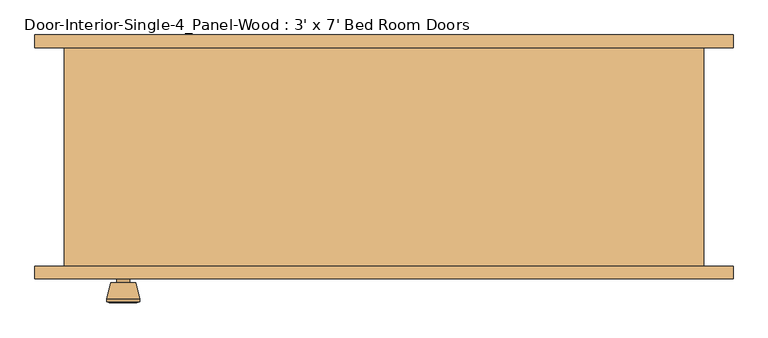
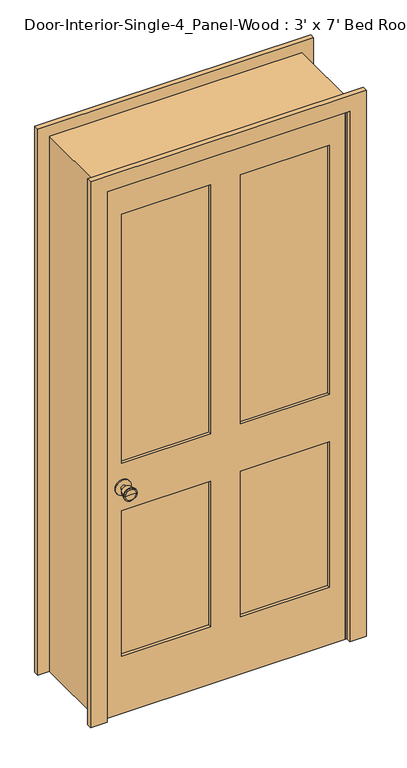
"""IFC4 building model written with IfcOpenShell, lengths in millimetres: door geometry, Door-Interior-Single-4_Panel-Wood : 3' x 7' Bed Room Doors."""

from ifc_helpers import new_model, si_unit, point, frame, frame_2d, origin, place, context, project, spatial, polyline, circle_curve, trimmed, segment, composite_curve, outline, extrude, faceted_brep, source, transform, mapped, element, save
from ifc_brep_helpers import plane_surface, cylinder_surface, revolved_surface, advanced_brep


def door_interior_single_4_panel_wood_3_x_7_bed_room_doors_8c54f457(model_context):
    return source(origin(), model_context, "Body", "SolidModel", [
        advanced_brep(
        [(-393.7, -121.0, 914.4), (-403.7, -121.0, 914.4), (-383.7, -121.0, 914.4), (-373.2241324, -72.0, 914.4), (-414.1758676, -72.0, 914.4), (-393.7, -72.0, 914.4), (-368.7, -73.8278681, 914.4), (-418.7, -73.8278681, 914.4), (-368.7, -77.2915463, 914.4), (-418.7, -77.2915463, 914.4), (-375.063764, -102.0, 914.4), (-412.336236, -102.0, 914.4), (-383.7, -102.0, 914.4), (-403.7, -102.0, 914.4)],
        [
            (0, 1),
            (1, 2, circle_curve(frame((-393.7, -121.0, 914.4), z_axis=(0.0, -1.0, 0.0), x_axis=(-1.0, 0.0, 0.0)), 10.0)),
            (2, 0),
            (2, 1, circle_curve(frame((-393.7, -121.0, 914.4), z_axis=(0.0, -1.0, 0.0), x_axis=(-1.0, 0.0, 0.0)), 10.0)),
            (3, 4, circle_curve(frame((-393.7, -72.0, 914.4), z_axis=(0.0, 1.0, 0.0), x_axis=(-1.0, 0.0, 0.0)), 20.4758676)),
            (4, 5),
            (5, 3),
            (4, 3, circle_curve(frame((-393.7, -72.0, 914.4), z_axis=(0.0, 1.0, 0.0), x_axis=(-1.0, 0.0, 0.0)), 20.4758676)),
            (6, 7, circle_curve(frame((-393.7, -73.8278681, 914.4), z_axis=(0.0, 1.0, 0.0), x_axis=(-1.0, 0.0, 0.0)), 25.0)),
            (7, 4),
            (3, 6),
            (7, 6, circle_curve(frame((-393.7, -73.8278681, 914.4), z_axis=(0.0, 1.0, 0.0), x_axis=(-1.0, 0.0, 0.0)), 25.0)),
            (8, 9, circle_curve(frame((-393.7, -77.2915463, 914.4), z_axis=(0.0, 1.0, 0.0), x_axis=(-1.0, 0.0, 0.0)), 25.0)),
            (9, 7),
            (6, 8),
            (9, 8, circle_curve(frame((-393.7, -77.2915463, 914.4), z_axis=(0.0, 1.0, 0.0), x_axis=(-1.0, 0.0, 0.0)), 25.0)),
            (10, 11, circle_curve(frame((-393.7, -102.0, 914.4), z_axis=(0.0, 1.0, 0.0), x_axis=(-1.0, 0.0, 0.0)), 18.636236)),
            (11, 9),
            (8, 10),
            (11, 10, circle_curve(frame((-393.7, -102.0, 914.4), z_axis=(0.0, 1.0, 0.0), x_axis=(-1.0, 0.0, 0.0)), 18.636236)),
            (12, 13, circle_curve(frame((-393.7, -102.0, 914.4), z_axis=(0.0, 1.0, 0.0), x_axis=(-1.0, 0.0, 0.0)), 10.0)),
            (13, 11),
            (10, 12),
            (13, 12, circle_curve(frame((-393.7, -102.0, 914.4), z_axis=(0.0, 1.0, 0.0), x_axis=(-1.0, 0.0, 0.0)), 10.0)),
            (1, 13),
            (12, 2),
        ],
        [
            plane_surface(frame((-393.7, -121.0, 914.4), z_axis=(0.0, -1.0, 0.0), x_axis=(-1.0, 0.0, 0.0))),
            plane_surface(frame((-393.7, -72.0, 914.4), z_axis=(0.0, 1.0, 0.0), x_axis=(-1.0, 0.0, 0.0))),
            revolved_surface(polyline([(-414.1758676, -72.0, 914.4), (-418.7, -73.8278681, 914.4)]), (-393.7, -121.0, 914.4), (0.0, -1.0, 0.0)),
            cylinder_surface(frame((-393.7, -121.0, 914.4), z_axis=(0.0, -1.0, 0.0), x_axis=(-1.0, 0.0, 0.0)), 25.0),
            revolved_surface(polyline([(-418.7, -77.2915463, 914.4), (-412.336236, -102.0, 914.4)]), (-393.7, -121.0, 914.4), (0.0, -1.0, 0.0)),
            plane_surface(frame((-393.7, -102.0, 914.4), z_axis=(0.0, -1.0, 0.0), x_axis=(-1.0, 0.0, 0.0))),
            cylinder_surface(frame((-393.7, -121.0, 914.4), z_axis=(0.0, -1.0, 0.0), x_axis=(-1.0, 0.0, 0.0)), 10.0),
        ],
        [
            (0, [[1, 2, 3]]),
            (0, [[-3, 4, -1]]),
            (1, [[5, 6, 7]]),
            (1, [[8, -7, -6]]),
            (2, [[9, 10, -5, 11]]),
            (2, [[12, -11, -8, -10]]),
            (3, [[13, 14, -9, 15]]),
            (3, [[16, -15, -12, -14]]),
            (4, [[17, 18, -13, 19]]),
            (4, [[20, -19, -16, -18]]),
            (5, [[21, 22, -17, 23]]),
            (5, [[24, -23, -20, -22]]),
            (6, [[-2, 25, -21, 26]]),
            (6, [[-4, -26, -24, -25]]),
        ],
    ),
        extrude(outline(composite_curve([segment(trimmed(circle_curve(frame_2d((914.4, -393.7)), 30.0), [point((914.4, -423.7))], [point((914.4, -363.7))], False, "CARTESIAN"), True, "CONTINUOUS"), segment(trimmed(circle_curve(frame_2d((914.4, -393.7)), 30.0), [point((914.4, -363.7))], [point((914.4, -423.7))], False, "CARTESIAN"), True, "CONTINUOUS")], self_intersect=False)), frame((0.0, -127.0, 0.0), z_axis=(0.0, 1.0, 0.0), x_axis=(0.0, 0.0, 1.0)), (0.0, 0.0, 1.0), 6.0),
        advanced_brep(
        [(-393.7, -167.925, 914.4), (-383.7, -167.925, 914.4), (-403.7, -167.925, 914.4), (-373.2241324, -216.925, 914.4), (-393.7, -216.925, 914.4), (-414.1758676, -216.925, 914.4), (-368.7, -215.0971319, 914.4), (-418.7, -215.0971319, 914.4), (-368.7, -211.6334537, 914.4), (-418.7, -211.6334537, 914.4), (-375.063764, -186.925, 914.4), (-412.336236, -186.925, 914.4), (-383.7, -186.925, 914.4), (-403.7, -186.925, 914.4)],
        [
            (0, 1),
            (1, 2, circle_curve(frame((-393.7, -167.925, 914.4), z_axis=(0.0, 1.0, 0.0), x_axis=(-1.0, 0.0, 0.0)), 10.0)),
            (2, 0),
            (2, 1, circle_curve(frame((-393.7, -167.925, 914.4), z_axis=(0.0, 1.0, 0.0), x_axis=(-1.0, 0.0, 0.0)), 10.0)),
            (3, 4),
            (4, 5),
            (5, 3, circle_curve(frame((-393.7, -216.925, 914.4), z_axis=(0.0, -1.0, 0.0), x_axis=(-1.0, 0.0, 0.0)), 20.4758676)),
            (3, 5, circle_curve(frame((-393.7, -216.925, 914.4), z_axis=(0.0, -1.0, 0.0), x_axis=(-1.0, 0.0, 0.0)), 20.4758676)),
            (6, 3),
            (5, 7),
            (7, 6, circle_curve(frame((-393.7, -215.0971319, 914.4), z_axis=(0.0, -1.0, 0.0), x_axis=(-1.0, 0.0, 0.0)), 25.0)),
            (6, 7, circle_curve(frame((-393.7, -215.0971319, 914.4), z_axis=(0.0, -1.0, 0.0), x_axis=(-1.0, 0.0, 0.0)), 25.0)),
            (8, 6),
            (7, 9),
            (9, 8, circle_curve(frame((-393.7, -211.6334537, 914.4), z_axis=(0.0, -1.0, 0.0), x_axis=(-1.0, 0.0, 0.0)), 25.0)),
            (8, 9, circle_curve(frame((-393.7, -211.6334537, 914.4), z_axis=(0.0, -1.0, 0.0), x_axis=(-1.0, 0.0, 0.0)), 25.0)),
            (10, 8),
            (9, 11),
            (11, 10, circle_curve(frame((-393.7, -186.925, 914.4), z_axis=(0.0, -1.0, 0.0), x_axis=(-1.0, 0.0, 0.0)), 18.636236)),
            (10, 11, circle_curve(frame((-393.7, -186.925, 914.4), z_axis=(0.0, -1.0, 0.0), x_axis=(-1.0, 0.0, 0.0)), 18.636236)),
            (12, 10),
            (11, 13),
            (13, 12, circle_curve(frame((-393.7, -186.925, 914.4), z_axis=(0.0, -1.0, 0.0), x_axis=(-1.0, 0.0, 0.0)), 10.0)),
            (12, 13, circle_curve(frame((-393.7, -186.925, 914.4), z_axis=(0.0, -1.0, 0.0), x_axis=(-1.0, 0.0, 0.0)), 10.0)),
            (1, 12),
            (13, 2),
        ],
        [
            plane_surface(frame((-393.7, -167.925, 914.4), z_axis=(0.0, 1.0, 0.0), x_axis=(-1.0, 0.0, 0.0))),
            plane_surface(frame((-393.7, -216.925, 914.4), z_axis=(0.0, -1.0, 0.0), x_axis=(-1.0, 0.0, 0.0))),
            revolved_surface(polyline([(-414.1758676, -216.925, 914.4), (-418.7, -215.0971319, 914.4)]), (-393.7, -167.925, 914.4), (0.0, 1.0, 0.0)),
            cylinder_surface(frame((-393.7, -167.925, 914.4), z_axis=(0.0, 1.0, 0.0), x_axis=(-1.0, 0.0, 0.0)), 25.0),
            revolved_surface(polyline([(-418.7, -211.6334537, 914.4), (-412.336236, -186.925, 914.4)]), (-393.7, -167.925, 914.4), (0.0, 1.0, 0.0)),
            plane_surface(frame((-393.7, -186.925, 914.4), z_axis=(0.0, 1.0, 0.0), x_axis=(-1.0, 0.0, 0.0))),
            cylinder_surface(frame((-393.7, -167.925, 914.4), z_axis=(0.0, 1.0, 0.0), x_axis=(-1.0, 0.0, 0.0)), 10.0),
        ],
        [
            (0, [[1, 2, 3]]),
            (0, [[-3, 4, -1]]),
            (1, [[5, 6, 7]]),
            (1, [[-6, -5, 8]]),
            (2, [[9, -7, 10, 11]]),
            (2, [[-10, -8, -9, 12]]),
            (3, [[13, -11, 14, 15]]),
            (3, [[-14, -12, -13, 16]]),
            (4, [[17, -15, 18, 19]]),
            (4, [[-18, -16, -17, 20]]),
            (5, [[21, -19, 22, 23]]),
            (5, [[-22, -20, -21, 24]]),
            (6, [[25, -23, 26, -2]]),
            (6, [[-26, -24, -25, -4]]),
        ],
    ),
        extrude(outline(composite_curve([segment(trimmed(circle_curve(frame_2d((914.4, -393.7)), 30.0), [point((914.4, -423.7))], [point((914.4, -363.7))], False, "CARTESIAN"), True, "CONTINUOUS"), segment(trimmed(circle_curve(frame_2d((914.4, -393.7)), 30.0), [point((914.4, -363.7))], [point((914.4, -423.7))], False, "CARTESIAN"), True, "CONTINUOUS")], self_intersect=False)), frame((0.0, -167.925, 0.0), z_axis=(0.0, 1.0, 0.0), x_axis=(0.0, 0.0, 1.0)), (0.0, 0.0, 1.0), 6.0),
        faceted_brep([(482.6, -161.925, 0.0), (457.2, -161.925, 0.0), (457.2, -127.0, 0.0), (444.5, -127.0, 0.0), (444.5, -92.075, 0.0), (457.2, -92.075, 0.0), (457.2, 168.275, 0.0), (482.6, 168.275, 0.0), (482.6, 168.275, 2159.0), (482.6, -161.925, 2159.0), (457.2, 168.275, 2133.6), (-457.2, 168.275, 2133.6), (-457.2, 168.275, 0.0), (-482.6, 168.275, 0.0), (-482.6, 168.275, 2159.0), (457.2, -92.075, 2133.6), (444.5, -92.075, 2120.9), (-444.5, -92.075, 2120.9), (-444.5, -92.075, 0.0), (-457.2, -92.075, 0.0), (-457.2, -92.075, 2133.6), (444.5, -127.0, 2120.9), (457.2, -127.0, 2133.6), (-457.2, -127.0, 2133.6), (-457.2, -127.0, 0.0), (-444.5, -127.0, 0.0), (-444.5, -127.0, 2120.9), (457.2, -161.925, 2133.6), (-482.6, -161.925, 2159.0), (-482.6, -161.925, 0.0), (-457.2, -161.925, 0.0), (-457.2, -161.925, 2133.6)], [[[0, 1, 2, 3, 4, 5, 6, 7]], [[7, 8, 9, 0]], [[6, 10, 11, 12, 13, 14, 8, 7]], [[5, 15, 10, 6]], [[4, 16, 17, 18, 19, 20, 15, 5]], [[3, 21, 16, 4]], [[2, 22, 23, 24, 25, 26, 21, 3]], [[1, 27, 22, 2]], [[0, 9, 28, 29, 30, 31, 27, 1]], [[8, 14, 28, 9]], [[15, 20, 11, 10]], [[21, 26, 17, 16]], [[27, 31, 23, 22]], [[29, 13, 12, 19, 18, 25, 24, 30]], [[14, 13, 29, 28]], [[20, 19, 12, 11]], [[26, 25, 18, 17]], [[31, 30, 24, 23]]]),
        extrude(outline(polyline([(2133.6, -457.2), (0.0, -457.2), (0.0, 457.2), (2133.6, 457.2), (2133.6, -457.2)]), holes=[polyline([(2014.5375, 57.15), (2014.5375, 396.875), (1009.65, 396.875), (1009.65, 57.15), (2014.5375, 57.15)]), polyline([(1009.65, -57.15), (1009.65, -396.875), (2014.5375, -396.875), (2014.5375, -57.15), (1009.65, -57.15)]), polyline([(819.15, 57.15), (819.15, 396.875), (231.775, 396.875), (231.775, 57.15), (819.15, 57.15)]), polyline([(231.775, -57.15), (231.775, -396.875), (819.15, -396.875), (819.15, -57.15), (231.775, -57.15)])]), frame((0.0, -161.925, 0.0), z_axis=(0.0, 1.0, 0.0), x_axis=(0.0, 0.0, 1.0)), (0.0, 0.0, 1.0), 34.925),
        extrude(outline(polyline([(396.875, -138.6416667), (396.875, -150.2833333), (57.15, -150.2833333), (57.15, -138.6416667), (396.875, -138.6416667)])), frame((0.0, 0.0, 1009.65), z_axis=(0.0, 0.0, 1.0), x_axis=(1.0, 0.0, 0.0)), (0.0, 0.0, 1.0), 1004.8875),
        extrude(outline(polyline([(-57.15, -138.6416667), (-57.15, -150.2833333), (-396.875, -150.2833333), (-396.875, -138.6416667), (-57.15, -138.6416667)])), frame((0.0, 0.0, 1009.65), z_axis=(0.0, 0.0, 1.0), x_axis=(1.0, 0.0, 0.0)), (0.0, 0.0, 1.0), 1004.8875),
        extrude(outline(polyline([(396.875, -138.6416667), (396.875, -150.2833333), (57.15, -150.2833333), (57.15, -138.6416667), (396.875, -138.6416667)])), frame((0.0, 0.0, 231.775), z_axis=(0.0, 0.0, 1.0), x_axis=(1.0, 0.0, 0.0)), (0.0, 0.0, 1.0), 587.375),
        extrude(outline(polyline([(-57.15, -138.6416667), (-57.15, -150.2833333), (-396.875, -150.2833333), (-396.875, -138.6416667), (-57.15, -138.6416667)])), frame((0.0, 0.0, 231.775), z_axis=(0.0, 0.0, 1.0), x_axis=(1.0, 0.0, 0.0)), (0.0, 0.0, 1.0), 587.375),
        extrude(outline(polyline([(0.0, 527.05), (2203.45, 527.05), (2203.45, -527.05), (0.0, -527.05), (0.0, -463.55), (2139.95, -463.55), (2139.95, 463.55), (0.0, 463.55), (0.0, 527.05)])), frame((0.0, -180.975, 0.0), z_axis=(0.0, 1.0, 0.0), x_axis=(0.0, 0.0, 1.0)), (0.0, 0.0, 1.0), 19.05),
        extrude(outline(polyline([(0.0, 527.05), (2203.45, 527.05), (2203.45, -527.05), (0.0, -527.05), (0.0, -463.55), (2139.95, -463.55), (2139.95, 463.55), (0.0, 463.55), (0.0, 527.05)])), frame((0.0, 168.275, 0.0), z_axis=(0.0, 1.0, 0.0), x_axis=(0.0, 0.0, 1.0)), (0.0, 0.0, 1.0), 19.05),
    ])


if __name__ == "__main__":
    model = new_model("IFC4")
    model_context = context("Model", 3, world=origin())
    ifc_project = project(units=[si_unit("LENGTHUNIT", "METRE", prefix="MILLI")], contexts=[model_context])
    site = spatial("IfcSite", under=ifc_project)
    building = spatial("IfcBuilding", under=site)
    placement = place(None, origin())
    door_interior_single_4_panel_wood_3_x_7_bed_room_doors_shape = door_interior_single_4_panel_wood_3_x_7_bed_room_doors_8c54f457(model_context)
    element("IfcDoor", 1, ObjectType="Door-Interior-Single-4_Panel-Wood : 3' x 7' Bed Room Doors", at=placement, inside=building, context=model_context, shape_type="MappedRepresentation", body=[
        mapped(door_interior_single_4_panel_wood_3_x_7_bed_room_doors_shape, transform((0.0, 0.0, 0.0), x_axis=(1.0, 0.0, 0.0), y_axis=(0.0, 1.0, 0.0), z_axis=(0.0, 0.0, 1.0))),
    ])
    save(model, "model.ifc")

# Revit data of these elements
# Type "Door-Interior-Single-4_Panel-Wood : 3' x 7' Bed Room Doors"
#   Type Mark = "13"
#   Assembly Code = "C1020300"
#   Analytic Construction = "Wooden"
#   Top Rail = 0' - 4 11/16"
#   Thickness = 0' - 1 3/8"
#   Thermal Resistance (R) = 2.5876 (h·ft²·°F)/BTU
#   Swing Angle [instance default] = 90.00°
#   Stiles = 0' - 2 3/8"
#   Rough Width = 3' - 2"
#   Rough Height = 7' - 1"
#   Mullion = 0' - 4 1/2"
#   Lock Rail = 0' - 7 1/2"
#   Height = 7' - 0"
#   Width = 3' - 0"
#   Heat Transfer Coefficient (U) = 0.3865 BTU/(h·ft²·°F)
#   Bottom Rail = 0' - 9 1/8"
#   Trim Material = Cherry
#   Panel Material = Cherry
#   Frame Material = Cherry
#   Door Handle Material = Aluminum
#   Visual Light Transmittance = 0
#   Solar Heat Gain Coefficient = 0
#   Wall Closure = (empty or 0)
#   Function = (empty or 0)
# Element 1 (IfcDoor, "Door-Interior-Single-4_Panel-Wood : 3' x 7' Bed Room Doors")
#   Materials on its faces: "Cherry", "Aluminum"
# Materials
#   "Cherry": class "Wood", colour RGB 226 177 128, transparency 0, Description = "Prunus Serotina", Cost = 0
#   "Aluminum": class "Metal", colour RGB 247 247 247, transparency 0, Description = "Aluminum 6061", Cost = 0
